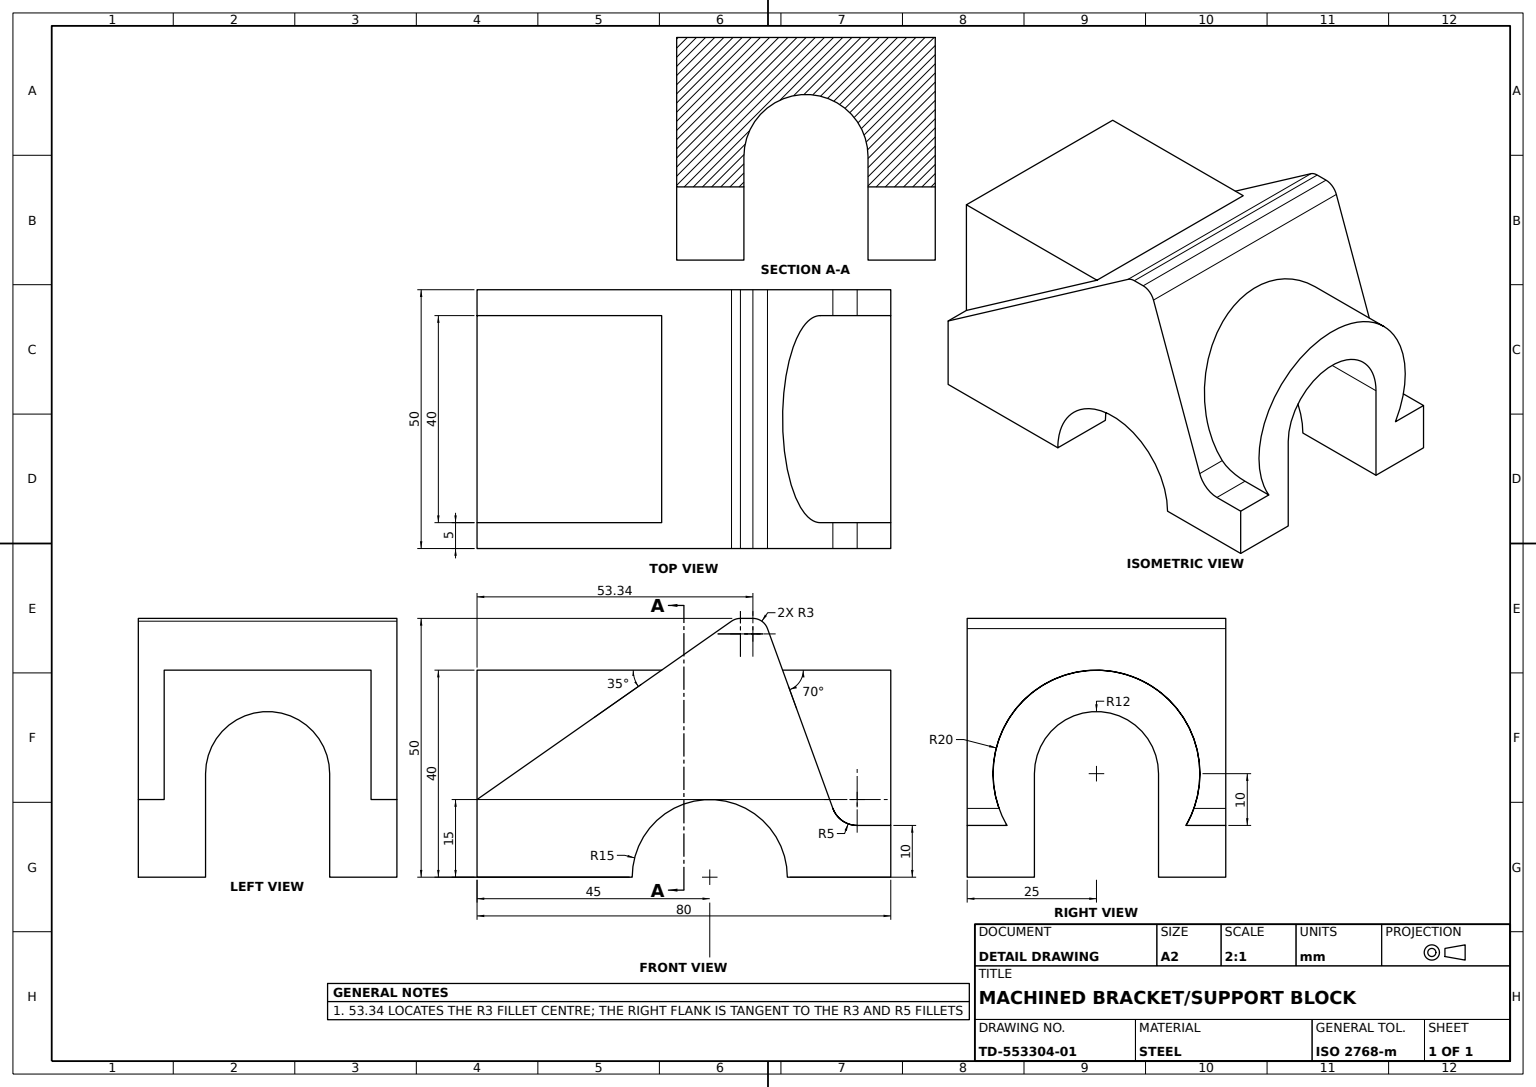
SolidWorks part; units mm, degrees
material "Plain Carbon Steel"
ref_plane "Front Plane" through (0, 0, 0) normal (0, 0, 1) x (1, 0, 0)
ref_plane "Top Plane" through (0, 0, 0) normal (0, 1, 0) x (1, 0, 0)
ref_plane "Right Plane" through (0, 0, 0) normal (1, 0, 0) x (0, 0, -1)
sketch "Base Profile Sketch" plane through (0, 0, 0) normal (1, 0, 0) x (0, 0, -1)
  line L0 (-17.3205, -10) -> (-25, -10)
  line L1 (-25, -10) -> (-25, -20)
  line L2 (-25, -20) -> (-12, -20)
  line L3 (0, -20) -> (0, 38.0732) construction
  line L4 (-12, 0) -> (-12, -20)
  line L5 (12, 0) -> (12, -20)
  line L6 (25, -10) -> (25, -20)
  line L7 (25, -20) -> (12, -20)
  line L8 (17.3205, -10) -> (25, -10)
  arc A0 (-17.3205, -10) -> (17.3205, -10) centre (0, 0) cw
  arc A1 (-12, 0) -> (12, 0) centre (0, 0) cw
  dimension "D1" = 20
  dimension "D4" = 12
  dimension "D2" = 10
  dimension "D3" = 20
  dimension "D5" = 24
  dimension "D6" = 50
extrude "Base Block" add sketch "Base Profile Sketch" against normal blind 25
sketch "Tower Sketch 40x40" plane through (-25, 0, 0) normal (-1, 0, 0) x (0, 0, 1)
  line L0 (-12, -20) -> (-25, -20) construction
  line L1 (-20, -20) -> (20, -20)
  line L2 (-20, -20) -> (-20, 20)
  line L3 (-20, 20) -> (20, 20)
  line L4 (20, -20) -> (20, 20)
  point P6 (0, -20)
  dimension "D1" = 40
  dimension "D2" = 40
extrude "Tower Block" add sketch "Tower Sketch 40x40" along normal blind 55
sketch "Ridge Profile Sketch" plane through (0, 0, 0) normal (0, 0, 1) x (1, 0, 0)
  line L0 (-80, -4.9974) -> (-30.0185, 30)
  line L1 (-80, -20) -> (-80, 20) construction
  line L2 (-30.0185, 30) -> (-24.56, 30)
  line L3 (-24.56, 30) -> (-10.0012, -10)
  line L5 (-80, 20) -> (0, 20) construction
  line L6 (-80, -4.9974) -> (-80, -20)
  line L7 (-80, -20) -> (0, -20)
  line L8 (0, -20) -> (0, -10)
  line L9 (0, -10) -> (-10.0012, -10)
  point P4 (-44.3, 20)
  point P10 (-44.3, 20)
  dimension "D1" = 35.7
  dimension "D2" = 50
  dimension "D3" = 145
  dimension "D4" = 110
  dimension "D5" = 55.44
extrude "Ridge Saddle Body" add sketch "Ridge Profile Sketch" along normal mid plane 50
fillet "Ridge Fillet R3" radius 3 2 edges at (-24.56, 30, 0) (-30.0185, 30, 0)
sketch "Saddle Opening Sketch" plane through (0, 0, 0) normal (1, 0, 0) x (0, 0, -1)
  line L0 (12, 0) -> (12, -10) construction
  line L1 (-12, -10) -> (-12, 0) construction
  line L2 (12, 0) -> (12, -10)
  line L3 (-12, -10) -> (-12, 0)
  line L4 (-12, -10) -> (-12, -20)
  line L5 (-25, -20) -> (25, -20) construction
  line L6 (-12, -20) -> (12, -20)
  line L7 (12, -20) -> (12, -10)
  arc A0 (12, 0) -> (-12, 0) centre (0, 0) ccw construction
  arc A1 (12, 0) -> (-12, 0) centre (0, 0) ccw
extrude "Saddle Opening Cut" cut sketch "Saddle Opening Sketch" against normal through all
sketch "Ridge Groove Sketch" plane through (0, 0, 25) normal (0, 0, 1) x (1, 0, 0)
  line L0 (-80, -20) -> (0, -20) construction
  line L1 (-80, -4.9974) -> (-80, -20) construction
  line L2 (-50, -20) -> (-20, -20)
  arc A0 (-50, -20) -> (-20, -20) centre (-35, -20) cw
  dimension "D1" = 15
  dimension "D2" = 45
extrude "Ridge Groove Cut" cut sketch "Ridge Groove Sketch" against normal through all
fillet "Edge Fillet R5" radius 5 2 edges at (-10.0012, -10, -21.1603) (-10.0012, -10, 21.1603)
